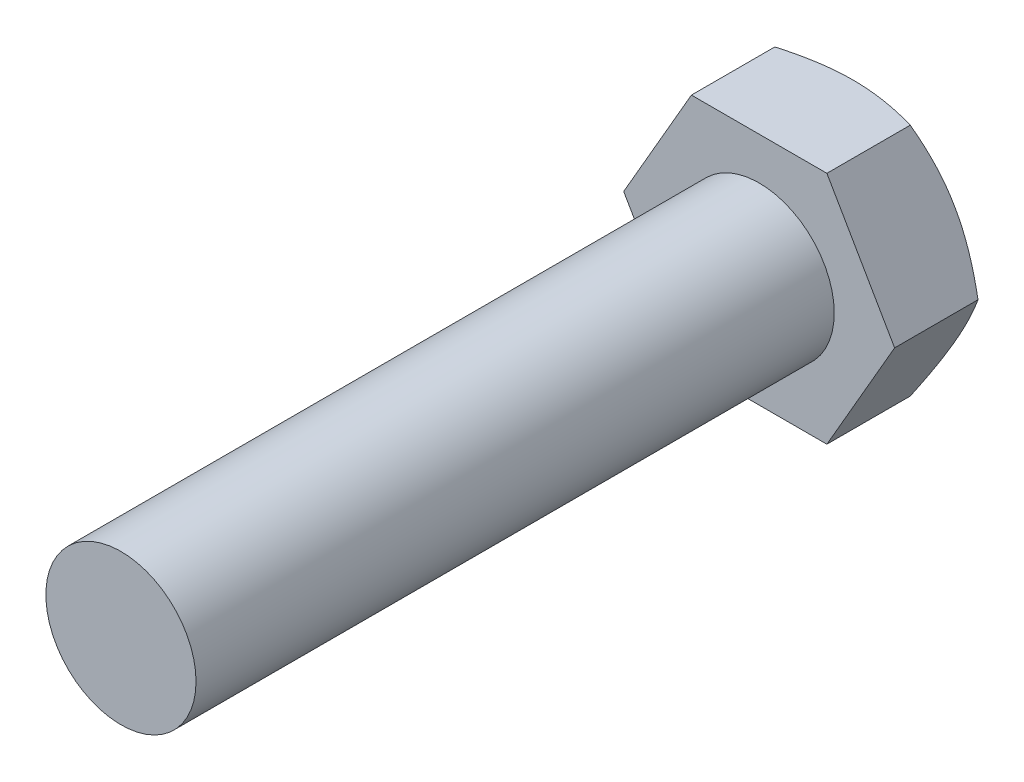
from build123d import *

# Parameters (mm, degrees)
HEX_HEAD_25AF_X10_DEPTH        = 10
HEAD_CHAMFER_PROFILE_OUTSIDE_W = 73.404
HEAD_CHAMFER_PROFILE_OUTSIDE_H = 69.536
HEAD_CHAMFER_PROFILE_OUTSIDE_R = 12.5
HEAD_CHAMFER_CUT_DEPTH         = 10
HEAD_CHAMFER_CUT_DRAFT         = -60
SHANK_PROFILE_16_R             = 8
SHANK_16_X68_DEPTH             = 68


with BuildPart() as part:
    # Hex Head Profile 25AF → Hex Head 25AF x10 (new body)
    with BuildSketch(Plane.XY):
        Polygon((14.43375673, 0), (7.216878365, 12.5), (-7.216878365, 12.5), (-14.43375673, 0), (-7.216878365, -12.5), (7.216878365, -12.5), align=None)
    extrude(amount=HEX_HEAD_25AF_X10_DEPTH)


with BuildPart() as head_chamfer_cut_tool:
    # Head Chamfer Profile outside → Head Chamfer Cut (with draft: the straight prism first)
    with BuildSketch(Plane(origin=(0, 0, 0), x_dir=(-1, 0, 0), z_dir=(0, 0, -1))):
        Rectangle(HEAD_CHAMFER_PROFILE_OUTSIDE_W, HEAD_CHAMFER_PROFILE_OUTSIDE_H)
        Circle(HEAD_CHAMFER_PROFILE_OUTSIDE_R, mode=Mode.SUBTRACT)
    extrude(amount=-HEAD_CHAMFER_CUT_DEPTH)
    # Head Chamfer Cut: the draft: its side faces are tilted about the plane it starts from
    head_chamfer_cut_sides = [head_chamfer_cut_tool.faces().sort_by_distance(p)[0] for p in [
        (0, -34.768, 5),
        (-36.702, 0, 5),
        (0, 34.768, 5),
        (36.702, 0, 5),
        (12.5, 0, 5),
    ]]
    draft(head_chamfer_cut_sides, Plane(origin=(0, 0, 0), x_dir=(-1, 0, 0), z_dir=(0, 0, -1)), HEAD_CHAMFER_CUT_DRAFT)


with BuildPart() as part_1:
    add(part.part)

    # Head Chamfer Cut: cut by head_chamfer_cut_tool
    add(head_chamfer_cut_tool.part, mode=Mode.SUBTRACT)

    # Shank Profile Ø16 → Shank Ø16 x68 (add)
    with BuildSketch(Plane.XY.offset(10)):
        Circle(SHANK_PROFILE_16_R)
    extrude(amount=SHANK_16_X68_DEPTH)


solid = part_1.part
